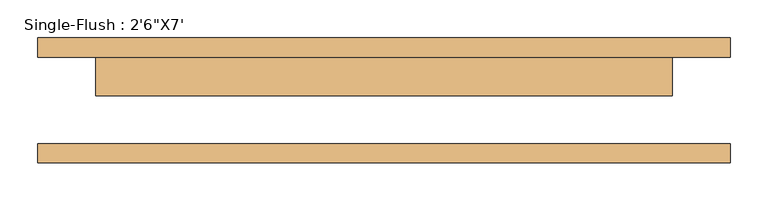
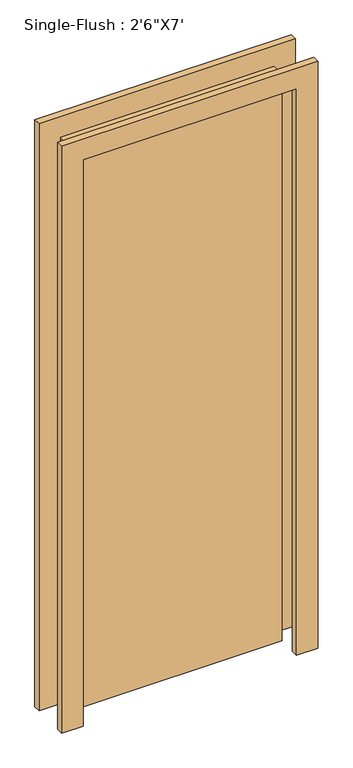
"""IFC4 building model written with IfcOpenShell, lengths in millimetres: door geometry."""

from ifc_helpers import new_model, si_unit, frame, origin, origin_with_axes, place, context, project, spatial, polyline, outline, extrude, source, transform, mapped, element, save


def door_214872d5(model_context):
    return source(origin(), model_context, "Body", "SweptSolid", [
        extrude(outline(polyline([(2209.8, -457.2), (0.0, -457.2), (0.0, -381.0), (2133.6, -381.0), (2133.6, 381.0), (0.0, 381.0), (0.0, 457.2), (2209.8, 457.2), (2209.8, -457.2)])), frame((0.0, 57.15, 0.0), z_axis=(0.0, 1.0, 0.0), x_axis=(0.0, 0.0, 1.0)), (0.0, 0.0, 1.0), 25.4),
        extrude(outline(polyline([(2209.8, 457.2), (2209.8, -457.2), (0.0, -457.2), (0.0, -381.0), (2133.6, -381.0), (2133.6, 381.0), (0.0, 381.0), (0.0, 457.2), (2209.8, 457.2)])), frame((0.0, -82.55, 0.0), z_axis=(0.0, 1.0, 0.0), x_axis=(0.0, 0.0, 1.0)), (0.0, 0.0, 1.0), 25.4),
        extrude(outline(polyline([(381.0, 6.35), (-381.0, 6.35), (-381.0, 57.15), (381.0, 57.15), (381.0, 6.35)])), origin_with_axes(), (0.0, 0.0, 1.0), 2133.6),
    ])


if __name__ == "__main__":
    model = new_model("IFC4")
    model_context = context("Model", 3, world=origin())
    ifc_project = project(units=[si_unit("LENGTHUNIT", "METRE", prefix="MILLI")], contexts=[model_context])
    site = spatial("IfcSite", under=ifc_project)
    building = spatial("IfcBuilding", under=site)
    placement = place(None, origin())
    door_shape = door_214872d5(model_context)
    element("IfcDoor", 1, ObjectType="Single-Flush : 2'6\"X7'", at=placement, inside=building, context=model_context, shape_type="MappedRepresentation", body=[
        mapped(door_shape, transform((0.0, 0.0, 0.0), x_axis=(1.0, 0.0, 0.0), y_axis=(0.0, 1.0, 0.0), z_axis=(0.0, 0.0, 1.0))),
    ])
    save(model, "model.ifc")

# Revit data of these elements
# Type "Single-Flush : 2'6\"X7'"
#   Type Mark = "9"
#   Construction Type Id = "MDOOR"
#   Assembly Code = "C1020"
#   Analytic Construction = "Metal"
#   Thickness = 0' - 2"
#   Heat Transfer Coefficient (U) = 0.651978 BTU/(h·ft²·°F)
#   Height = 7' - 0"
#   Trim Projection Ext = 0' - 1"
#   Trim Projection Int = 0' - 1"
#   Trim Width = 0' - 3"
#   Width = 2' - 6"
#   Define Thermal Properties by = 1
#   Door Material = Door - Panel
#   Frame Material = Door - Frame
#   Visual Light Transmittance = 0
#   Solar Heat Gain Coefficient = 0
#   Function = (empty or 0)
#   Wall Closure = (empty or 0)
# Element 1 (IfcDoor, "Single-Flush : 2'6\"X7'")
#   Materials on its faces: "Door - Frame", "Door - Panel"
# Materials
#   "Door - Panel": class "Wood", colour RGB 210 159 95, transparency 0, Cost = 0
#   "Door - Frame": colour RGB 118 70 51, transparency 0, Cost = 0
